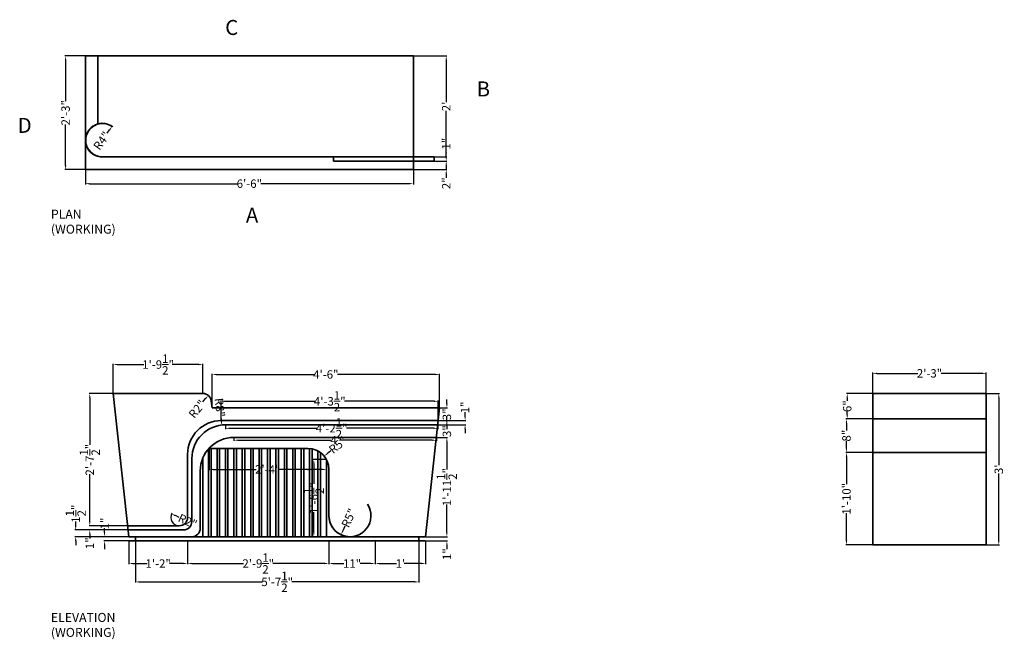
# Model space of a CAD drawing. Units: inches. Extents: x 461 to 695, y 519 to 666.
import ezdxf

# ---------------------------------------------------------------- set-up
doc = ezdxf.new("R2010")
doc.units = ezdxf.units.IN
doc.header["$MEASUREMENT"] = 0
for name, color, linetype, lineweight in [('A-ANNO-DIMS', 2, 'Continuous', 18), ('A-ANNO-TEXT', 3, 'Continuous', 25), ('A-FURN', 7, 'Continuous', 35)]:
    doc.layers.add(name, color=color, linetype=linetype, lineweight=lineweight)
doc.styles.get("Standard").update_dxf_attribs({"font": 'arial.ttf'})
doc.dimstyles.get("Standard").update_dxf_attribs({"dimtxt": 2, "dimasz": 1, "dimexe": 0.18, "dimexo": 0.0625, "dimgap": 0.09, "dimtad": 0, "dimdec": 1, "dimzin": 0, "dimdsep": 46, "dimlunit": 4, "dimtxsty": 'Standard', "dimcen": 0.09, "dimadec": 0, "dimazin": 0, "dimtfac": 1, "dimtdec": 1, "dimtofl": 0, "dimtmove": 0, "dimatfit": 3, "dimfxl": 1, "dimtolj": 1, "dimtzin": 0, "dimarcsym": 0})

# ---------------------------------------------------------------- blocks, each defined once
blk = doc.blocks.new('*D1')
at = {"layer": 'A-ANNO-DIMS', "color": 0, "lineweight": -2, "transparency": 16777216}
for p, q in [((562.35, 634.24), (562.35, 635.24)), ((559.57, 633.24), (562.53, 633.24)), ((559.57, 632.24), (562.53, 632.24)), ((562.35, 631.24), (562.35, 630.24))]:
    blk.add_line(p, q, dxfattribs=at)
at = {"layer": 'A-ANNO-DIMS', "color": 0, "transparency": 16777216}
for points in [[(562.18, 634.24), (562.51, 634.24), (562.35, 633.24)], [(562.18, 631.24), (562.51, 631.24), (562.35, 632.24)]]:
    blk.add_solid(points, dxfattribs=at)
at = {"layer": 'Defpoints', "color": 0, "transparency": 16777216}
for p in [(559.51, 633.24), (559.51, 632.24), (562.35, 633.24)]:
    blk.add_point(p, dxfattribs=at)
at = {"layer": 'A-ANNO-DIMS', "color": 0, "transparency": 16777216, "insert": (562.35, 636.39), "char_height": 2, "attachment_point": 5, "rotation": 90}
blk.add_mtext('\\A1;1"', dxfattribs=at)
blk = doc.blocks.new('*D2')
at = {"layer": 'A-ANNO-DIMS', "color": 0, "lineweight": -2, "transparency": 16777216}
for p, q in [((554.59, 632.24), (562.53, 632.24)), ((562.35, 633.24), (562.35, 634.24)), ((554.59, 630.24), (562.53, 630.24)), ((562.35, 629.24), (562.35, 628.24))]:
    blk.add_line(p, q, dxfattribs=at)
at = {"layer": 'A-ANNO-DIMS', "color": 0, "transparency": 16777216}
for points in [[(562.18, 633.24), (562.51, 633.24), (562.35, 632.24)], [(562.18, 629.24), (562.51, 629.24), (562.35, 630.24)]]:
    blk.add_solid(points, dxfattribs=at)
at = {"layer": 'Defpoints', "color": 0, "transparency": 16777216}
for p in [(554.53, 632.24), (554.53, 630.24), (562.35, 630.24)]:
    blk.add_point(p, dxfattribs=at)
at = {"layer": 'A-ANNO-DIMS', "color": 0, "transparency": 16777216, "insert": (562.35, 626.98), "char_height": 2, "attachment_point": 5, "rotation": 90}
blk.add_mtext('\\A1;2"', dxfattribs=at)
blk = doc.blocks.new('*D3')
at = {"layer": 'A-ANNO-DIMS', "color": 0, "lineweight": -2, "transparency": 16777216}
for p, q in [((554.59, 657.24), (562.53, 657.24)), ((562.35, 656.24), (562.35, 646.27)), ((562.35, 634.24), (562.35, 644.21)), ((554.59, 633.24), (562.53, 633.24))]:
    blk.add_line(p, q, dxfattribs=at)
at = {"layer": 'A-ANNO-DIMS', "color": 0, "transparency": 16777216}
for points in [[(562.18, 656.24), (562.51, 656.24), (562.35, 657.24)], [(562.18, 634.24), (562.51, 634.24), (562.35, 633.24)]]:
    blk.add_solid(points, dxfattribs=at)
at = {"layer": 'Defpoints', "color": 0, "transparency": 16777216}
for p in [(554.53, 657.24), (562.35, 657.24), (554.53, 633.24)]:
    blk.add_point(p, dxfattribs=at)
at = {"layer": 'A-ANNO-DIMS', "color": 0, "transparency": 16777216, "insert": (562.35, 645.24), "char_height": 2, "attachment_point": 5, "rotation": 90}
blk.add_mtext("\\A1;2'", dxfattribs=at)
blk = doc.blocks.new('*D4')
at = {"layer": 'A-ANNO-DIMS', "color": 0, "lineweight": -2, "transparency": 16777216}
for p, q in [((476.53, 630.18), (476.53, 626.7)), ((554.53, 630.18), (554.53, 626.7)), ((477.53, 626.88), (512.77, 626.88)), ((553.53, 626.88), (518.28, 626.88))]:
    blk.add_line(p, q, dxfattribs=at)
at = {"layer": 'A-ANNO-DIMS', "color": 0, "transparency": 16777216}
for points in [[(477.53, 627.04), (477.53, 626.71), (476.53, 626.88)], [(553.53, 627.04), (553.53, 626.71), (554.53, 626.88)]]:
    blk.add_solid(points, dxfattribs=at)
at = {"layer": 'Defpoints', "color": 0, "transparency": 16777216}
for p in [(476.53, 630.24), (554.53, 630.24), (476.53, 626.88)]:
    blk.add_point(p, dxfattribs=at)
at = {"layer": 'A-ANNO-DIMS', "color": 0, "transparency": 16777216, "insert": (515.53, 626.88), "char_height": 2, "attachment_point": 5}
blk.add_mtext('\\A1;6\'-6"', dxfattribs=at)
blk = doc.blocks.new('*D5')
at = {"layer": 'A-ANNO-DIMS', "color": 0, "lineweight": -2, "transparency": 16777216}
for p, q in [((476.46, 657.24), (471.65, 657.24)), ((471.83, 656.24), (471.83, 646.51)), ((471.83, 631.24), (471.83, 640.98)), ((476.46, 630.24), (471.65, 630.24))]:
    blk.add_line(p, q, dxfattribs=at)
at = {"layer": 'A-ANNO-DIMS', "color": 0, "transparency": 16777216}
for points in [[(471.66, 656.24), (472, 656.24), (471.83, 657.24)], [(471.66, 631.24), (472, 631.24), (471.83, 630.24)]]:
    blk.add_solid(points, dxfattribs=at)
at = {"layer": 'Defpoints', "color": 0, "transparency": 16777216}
for p in [(476.53, 657.24), (471.83, 630.24), (476.53, 630.24)]:
    blk.add_point(p, dxfattribs=at)
at = {"layer": 'A-ANNO-DIMS', "color": 0, "transparency": 16777216, "insert": (471.83, 643.74), "char_height": 2, "attachment_point": 5, "rotation": 90}
blk.add_mtext('\\A1;2\'-3"', dxfattribs=at)
blk = doc.blocks.new('*D6')
at = {"layer": 'A-ANNO-DIMS', "color": 0, "lineweight": -2, "transparency": 16777216}
blk.add_line((481.7, 638.86), (482.29, 639.67), dxfattribs=at)
blk.add_arc((480.53, 637.24), 4, 51.3987, 179.1048, dxfattribs=at)
at = {"layer": 'A-ANNO-DIMS', "color": 0, "transparency": 16777216}
blk.add_solid([(482.16, 639.76), (482.43, 639.57), (482.88, 640.48)], dxfattribs=at)
at = {"layer": 'Defpoints', "color": 0, "transparency": 16777216}
for p in [(482.88, 640.48), (480.53, 637.24)]:
    blk.add_point(p, dxfattribs=at)
at = {"layer": 'A-ANNO-DIMS', "color": 0, "transparency": 16777216, "insert": (480.41, 637.08), "char_height": 2, "attachment_point": 5, "rotation": 53.977}
blk.add_mtext('\\A1;R4"', dxfattribs=at)
blk = doc.blocks.new('*D7')
at = {"layer": 'A-ANNO-DIMS', "color": 0, "lineweight": -2, "transparency": 16777216}
for p, q in [((500.85, 541.88), (500.85, 536.4)), ((534.45, 541.88), (534.45, 536.4)), ((501.85, 536.58), (514.16, 536.58)), ((533.45, 536.58), (521.15, 536.58))]:
    blk.add_line(p, q, dxfattribs=at)
at = {"layer": 'A-ANNO-DIMS', "color": 0, "transparency": 16777216}
for points in [[(501.85, 536.74), (501.85, 536.41), (500.85, 536.58)], [(533.45, 536.74), (533.45, 536.41), (534.45, 536.58)]]:
    blk.add_solid(points, dxfattribs=at)
at = {"layer": 'Defpoints', "color": 0, "transparency": 16777216}
for p in [(500.85, 541.95), (534.45, 541.95), (534.45, 536.58)]:
    blk.add_point(p, dxfattribs=at)
at = {"layer": 'A-ANNO-DIMS', "color": 0, "transparency": 16777216, "insert": (517.65, 536.58), "char_height": 2, "attachment_point": 5}
blk.add_mtext('\\A1;2\'-9{\\H1x;\\S1/2;}"', dxfattribs=at)
blk = doc.blocks.new('*D8')
at = {"layer": 'A-ANNO-DIMS', "color": 0, "lineweight": -2, "transparency": 16777216}
for p, q in [((486.85, 541.88), (486.85, 536.4)), ((500.85, 541.88), (500.85, 536.4)), ((487.85, 536.58), (491.2, 536.58)), ((499.85, 536.58), (496.51, 536.58))]:
    blk.add_line(p, q, dxfattribs=at)
at = {"layer": 'A-ANNO-DIMS', "color": 0, "transparency": 16777216}
for points in [[(487.85, 536.74), (487.85, 536.41), (486.85, 536.58)], [(499.85, 536.74), (499.85, 536.41), (500.85, 536.58)]]:
    blk.add_solid(points, dxfattribs=at)
at = {"layer": 'Defpoints', "color": 0, "transparency": 16777216}
for p in [(486.85, 541.95), (500.85, 541.95), (500.85, 536.58)]:
    blk.add_point(p, dxfattribs=at)
at = {"layer": 'A-ANNO-DIMS', "color": 0, "transparency": 16777216, "insert": (493.85, 536.58), "char_height": 2, "attachment_point": 5}
blk.add_mtext('\\A1;1\'-2"', dxfattribs=at)
blk = doc.blocks.new('*D9')
at = {"layer": 'A-ANNO-DIMS', "color": 0, "lineweight": -2, "transparency": 16777216}
for p, q in [((534.45, 541.88), (534.45, 536.4)), ((545.45, 541.88), (545.45, 536.4)), ((535.45, 536.58), (538.03, 536.58)), ((544.45, 536.58), (541.87, 536.58))]:
    blk.add_line(p, q, dxfattribs=at)
at = {"layer": 'A-ANNO-DIMS', "color": 0, "transparency": 16777216}
for points in [[(535.45, 536.74), (535.45, 536.41), (534.45, 536.58)], [(544.45, 536.74), (544.45, 536.41), (545.45, 536.58)]]:
    blk.add_solid(points, dxfattribs=at)
at = {"layer": 'Defpoints', "color": 0, "transparency": 16777216}
for p in [(534.45, 541.95), (545.45, 541.95), (545.45, 536.58)]:
    blk.add_point(p, dxfattribs=at)
at = {"layer": 'A-ANNO-DIMS', "color": 0, "transparency": 16777216, "insert": (539.95, 536.58), "char_height": 2, "attachment_point": 5}
blk.add_mtext('\\A1;11"', dxfattribs=at)
blk = doc.blocks.new('*D10')
at = {"layer": 'A-ANNO-DIMS', "color": 0, "lineweight": -2, "transparency": 16777216}
for p, q in [((545.45, 541.88), (545.45, 536.4)), ((557.45, 541.88), (557.45, 536.4)), ((546.45, 536.58), (550.54, 536.58)), ((556.45, 536.58), (552.37, 536.58))]:
    blk.add_line(p, q, dxfattribs=at)
at = {"layer": 'A-ANNO-DIMS', "color": 0, "transparency": 16777216}
for points in [[(546.45, 536.74), (546.45, 536.41), (545.45, 536.58)], [(556.45, 536.74), (556.45, 536.41), (557.45, 536.58)]]:
    blk.add_solid(points, dxfattribs=at)
at = {"layer": 'Defpoints', "color": 0, "transparency": 16777216}
for p in [(545.45, 541.95), (557.45, 541.95), (557.45, 536.58)]:
    blk.add_point(p, dxfattribs=at)
at = {"layer": 'A-ANNO-DIMS', "color": 0, "transparency": 16777216, "insert": (551.45, 536.58), "char_height": 2, "attachment_point": 5}
blk.add_mtext("\\A1;1'", dxfattribs=at)
blk = doc.blocks.new('*D11')
at = {"layer": 'A-ANNO-DIMS', "color": 0, "lineweight": -2, "transparency": 16777216}
blk.add_line((498.85, 547.55), (497.94, 547.96), dxfattribs=at)
blk.add_arc((498.85, 547.55), 2, 150.5064, 268.2095, dxfattribs=at)
at = {"layer": 'A-ANNO-DIMS', "color": 0, "transparency": 16777216}
blk.add_solid([(498.01, 548.11), (497.87, 547.81), (497.03, 548.37)], dxfattribs=at)
at = {"layer": 'Defpoints', "color": 0, "transparency": 16777216}
for p in [(497.03, 548.37), (498.85, 547.55)]:
    blk.add_point(p, dxfattribs=at)
at = {"layer": 'A-ANNO-DIMS', "color": 0, "transparency": 16777216, "insert": (500.85, 546.64), "char_height": 2, "attachment_point": 5, "rotation": 335.663}
blk.add_mtext('\\A1;R2"', dxfattribs=at)
blk = doc.blocks.new('*D12')
at = {"layer": 'A-ANNO-DIMS', "color": 0, "lineweight": -2, "transparency": 16777216}
blk.add_line((538.27, 545.42), (537.76, 544.32), dxfattribs=at)
at = {"layer": 'A-ANNO-DIMS', "color": 0, "transparency": 16777216}
blk.add_solid([(537.61, 544.39), (537.91, 544.25), (537.34, 543.42)], dxfattribs=at)
at = {"layer": 'Defpoints', "color": 0, "transparency": 16777216}
for p in [(539.45, 547.95), (537.34, 543.42)]:
    blk.add_point(p, dxfattribs=at)
at = {"layer": 'A-ANNO-DIMS', "color": 0, "transparency": 16777216, "insert": (539.2, 547.41), "char_height": 2, "attachment_point": 5, "rotation": 65.0007}
blk.add_mtext('\\A1;R5"', dxfattribs=at)
blk = doc.blocks.new('*D13')
at = {"layer": 'A-ANNO-DIMS', "color": 0, "lineweight": -2, "transparency": 16777216}
for p, q in [((508.75, 571.49), (508.86, 570.49)), ((509.76, 561.55), (509.94, 561.55)), ((509.85, 561.46), (509.85, 561.64))]:
    blk.add_line(p, q, dxfattribs=at)
at = {"layer": 'A-ANNO-DIMS', "color": 0, "transparency": 16777216}
blk.add_solid([(509.02, 570.51), (508.69, 570.47), (508.97, 569.5)], dxfattribs=at)
at = {"layer": 'Defpoints', "color": 0, "transparency": 16777216}
for p in [(508.97, 569.5), (509.85, 561.55)]:
    blk.add_point(p, dxfattribs=at)
at = {"layer": 'A-ANNO-DIMS', "color": 0, "transparency": 16777216, "insert": (508.51, 573.67), "char_height": 2, "attachment_point": 5, "rotation": 276.3402}
blk.add_mtext('\\A1;R8"', dxfattribs=at)
blk = doc.blocks.new('*D14')
at = {"layer": 'A-ANNO-DIMS', "color": 0, "lineweight": -2, "transparency": 16777216}
blk.add_line((504.49, 575), (505.12, 575.78), dxfattribs=at)
at = {"layer": 'A-ANNO-DIMS', "color": 0, "transparency": 16777216}
blk.add_solid([(505, 575.88), (505.25, 575.67), (505.76, 576.55)], dxfattribs=at)
at = {"layer": 'Defpoints', "color": 0, "transparency": 16777216}
for p in [(505.76, 576.55), (504.49, 575)]:
    blk.add_point(p, dxfattribs=at)
at = {"layer": 'A-ANNO-DIMS', "color": 0, "transparency": 16777216, "insert": (503.11, 573.3), "char_height": 2, "attachment_point": 5, "rotation": 50.8113}
blk.add_mtext('\\A1;R2"', dxfattribs=at)
blk = doc.blocks.new('*D15')
at = {"layer": 'A-ANNO-DIMS', "color": 0, "lineweight": -2, "transparency": 16777216}
for p, q in [((534.89, 563.36), (534.11, 562.73)), ((529.36, 558.95), (529.54, 558.95)), ((529.45, 558.86), (529.45, 559.04))]:
    blk.add_line(p, q, dxfattribs=at)
at = {"layer": 'A-ANNO-DIMS', "color": 0, "transparency": 16777216}
blk.add_solid([(534, 562.86), (534.21, 562.6), (533.33, 562.1)], dxfattribs=at)
at = {"layer": 'Defpoints', "color": 0, "transparency": 16777216}
for p in [(533.33, 562.1), (529.45, 558.95)]:
    blk.add_point(p, dxfattribs=at)
at = {"layer": 'A-ANNO-DIMS', "color": 0, "transparency": 16777216, "insert": (536.59, 564.75), "char_height": 2, "attachment_point": 5, "rotation": 39.0868}
blk.add_mtext('\\A1;R5"', dxfattribs=at)
blk = doc.blocks.new('*D16')
at = {"layer": 'A-ANNO-DIMS', "color": 0, "lineweight": -2, "transparency": 16777216}
for p, q in [((506.66, 573.61), (506.66, 581.7)), ((507.66, 581.52), (530.93, 581.52)), ((559.78, 581.52), (536.51, 581.52)), ((560.78, 573.61), (560.78, 581.7))]:
    blk.add_line(p, q, dxfattribs=at)
at = {"layer": 'A-ANNO-DIMS', "color": 0, "transparency": 16777216}
for points in [[(507.66, 581.68), (507.66, 581.35), (506.66, 581.52)], [(559.78, 581.68), (559.78, 581.35), (560.78, 581.52)]]:
    blk.add_solid(points, dxfattribs=at)
at = {"layer": 'Defpoints', "color": 0, "transparency": 16777216}
for p in [(506.66, 581.52), (506.66, 573.55), (560.78, 573.55)]:
    blk.add_point(p, dxfattribs=at)
at = {"layer": 'A-ANNO-DIMS', "color": 0, "transparency": 16777216, "insert": (533.72, 581.52), "char_height": 2, "attachment_point": 5}
blk.add_mtext('\\A1;4\'-6"', dxfattribs=at)
blk = doc.blocks.new('*D17')
at = {"layer": 'A-ANNO-DIMS', "color": 0, "lineweight": -2, "transparency": 16777216}
for p, q in [((483.15, 577.06), (483.15, 584.06)), ((484.15, 583.88), (490.44, 583.88)), ((503.49, 583.88), (497.21, 583.88)), ((504.49, 577.06), (504.49, 584.06))]:
    blk.add_line(p, q, dxfattribs=at)
at = {"layer": 'A-ANNO-DIMS', "color": 0, "transparency": 16777216}
for points in [[(484.15, 584.05), (484.15, 583.72), (483.15, 583.88)], [(503.49, 584.05), (503.49, 583.72), (504.49, 583.88)]]:
    blk.add_solid(points, dxfattribs=at)
at = {"layer": 'Defpoints', "color": 0, "transparency": 16777216}
for p in [(504.49, 583.88), (483.15, 577), (504.49, 577)]:
    blk.add_point(p, dxfattribs=at)
at = {"layer": 'A-ANNO-DIMS', "color": 0, "transparency": 16777216, "insert": (493.82, 583.88), "char_height": 2, "attachment_point": 5}
blk.add_mtext('\\A1;1\'-9{\\H1x;\\S1/2;}"', dxfattribs=at)
blk = doc.blocks.new('*D18')
at = {"layer": 'A-ANNO-DIMS', "color": 0, "lineweight": -2, "transparency": 16777216}
for p, q in [((562.5, 543.95), (562.5, 544.95)), ((557.41, 541.95), (562.68, 541.95)), ((557.51, 542.95), (562.68, 542.95)), ((562.5, 540.95), (562.5, 539.95))]:
    blk.add_line(p, q, dxfattribs=at)
at = {"layer": 'A-ANNO-DIMS', "color": 0, "transparency": 16777216}
for points in [[(562.34, 543.95), (562.67, 543.95), (562.5, 542.95)], [(562.34, 540.95), (562.67, 540.95), (562.5, 541.95)]]:
    blk.add_solid(points, dxfattribs=at)
at = {"layer": 'Defpoints', "color": 0, "transparency": 16777216}
for p in [(557.34, 541.95), (557.45, 542.95), (562.5, 541.95)]:
    blk.add_point(p, dxfattribs=at)
at = {"layer": 'A-ANNO-DIMS', "color": 0, "transparency": 16777216, "insert": (562.5, 538.8), "char_height": 2, "attachment_point": 5, "rotation": 90}
blk.add_mtext('\\A1;1"', dxfattribs=at)
blk = doc.blocks.new('*D19')
at = {"layer": 'A-ANNO-DIMS', "color": 0, "lineweight": -2, "transparency": 16777216}
for p, q in [((560.08, 566.55), (562.68, 566.55)), ((562.5, 565.55), (562.5, 558.91)), ((562.5, 543.95), (562.5, 550.59)), ((557.51, 542.95), (562.68, 542.95))]:
    blk.add_line(p, q, dxfattribs=at)
at = {"layer": 'A-ANNO-DIMS', "color": 0, "transparency": 16777216}
for points in [[(562.34, 565.55), (562.67, 565.55), (562.5, 566.55)], [(562.34, 543.95), (562.67, 543.95), (562.5, 542.95)]]:
    blk.add_solid(points, dxfattribs=at)
at = {"layer": 'Defpoints', "color": 0, "transparency": 16777216}
for p in [(560.02, 566.55), (562.5, 566.55), (557.45, 542.95)]:
    blk.add_point(p, dxfattribs=at)
at = {"layer": 'A-ANNO-DIMS', "color": 0, "transparency": 16777216, "insert": (562.5, 554.75), "char_height": 2, "attachment_point": 5, "rotation": 90}
blk.add_mtext('\\A1;1\'-11{\\H1x;\\S1/2;}"', dxfattribs=at)
blk = doc.blocks.new('*D20')
at = {"layer": 'A-ANNO-DIMS', "color": 0, "lineweight": -2, "transparency": 16777216}
for p, q in [((562.5, 570.55), (562.5, 571.55)), ((560.4, 569.55), (562.68, 569.55)), ((560.08, 566.55), (562.68, 566.55)), ((562.5, 565.55), (562.5, 564.55))]:
    blk.add_line(p, q, dxfattribs=at)
at = {"layer": 'A-ANNO-DIMS', "color": 0, "transparency": 16777216}
for points in [[(562.34, 570.55), (562.67, 570.55), (562.5, 569.55)], [(562.34, 565.55), (562.67, 565.55), (562.5, 566.55)]]:
    blk.add_solid(points, dxfattribs=at)
at = {"layer": 'Defpoints', "color": 0, "transparency": 16777216}
for p in [(560.34, 569.55), (560.02, 566.55), (562.5, 566.55)]:
    blk.add_point(p, dxfattribs=at)
at = {"layer": 'A-ANNO-DIMS', "color": 0, "transparency": 16777216, "insert": (562.5, 568.05), "char_height": 2, "attachment_point": 5, "rotation": 90}
blk.add_mtext('\\A1;3"', dxfattribs=at)
blk = doc.blocks.new('*D21')
at = {"layer": 'A-ANNO-DIMS', "color": 0, "lineweight": -2, "transparency": 16777216}
for p, q in [((566.83, 571.55), (566.83, 572.55)), ((560.4, 569.55), (567.01, 569.55)), ((560.51, 570.55), (567.01, 570.55)), ((566.83, 568.55), (566.83, 567.55))]:
    blk.add_line(p, q, dxfattribs=at)
at = {"layer": 'A-ANNO-DIMS', "color": 0, "transparency": 16777216}
for points in [[(566.67, 571.55), (567, 571.55), (566.83, 570.55)], [(566.67, 568.55), (567, 568.55), (566.83, 569.55)]]:
    blk.add_solid(points, dxfattribs=at)
at = {"layer": 'Defpoints', "color": 0, "transparency": 16777216}
for p in [(560.34, 569.55), (560.45, 570.55), (566.83, 570.55)]:
    blk.add_point(p, dxfattribs=at)
at = {"layer": 'A-ANNO-DIMS', "color": 0, "transparency": 16777216, "insert": (566.83, 573.69), "char_height": 2, "attachment_point": 5, "rotation": 90}
blk.add_mtext('\\A1;1"', dxfattribs=at)
blk = doc.blocks.new('*D22')
at = {"layer": 'A-ANNO-DIMS', "color": 0, "lineweight": -2, "transparency": 16777216}
for p, q in [((562.5, 574.55), (562.5, 575.55)), ((560.84, 573.55), (562.68, 573.55)), ((560.51, 570.55), (562.68, 570.55)), ((562.5, 569.55), (562.5, 568.55))]:
    blk.add_line(p, q, dxfattribs=at)
at = {"layer": 'A-ANNO-DIMS', "color": 0, "transparency": 16777216}
for points in [[(562.34, 574.55), (562.67, 574.55), (562.5, 573.55)], [(562.34, 569.55), (562.67, 569.55), (562.5, 570.55)]]:
    blk.add_solid(points, dxfattribs=at)
at = {"layer": 'Defpoints', "color": 0, "transparency": 16777216}
for p in [(560.78, 573.55), (560.45, 570.55), (562.5, 570.55)]:
    blk.add_point(p, dxfattribs=at)
at = {"layer": 'A-ANNO-DIMS', "color": 0, "transparency": 16777216, "insert": (562.5, 572.05), "char_height": 2, "attachment_point": 5, "rotation": 90}
blk.add_mtext('\\A1;3"', dxfattribs=at)
blk = doc.blocks.new('*D23')
at = {"layer": 'A-ANNO-DIMS', "color": 0, "lineweight": -2, "transparency": 16777216}
for p, q in [((481.09, 543.95), (481.09, 544.95)), ((486.79, 542.95), (480.91, 542.95)), ((486.9, 541.95), (480.91, 541.95)), ((481.09, 540.95), (481.09, 539.95))]:
    blk.add_line(p, q, dxfattribs=at)
at = {"layer": 'A-ANNO-DIMS', "color": 0, "transparency": 16777216}
for points in [[(480.93, 543.95), (481.26, 543.95), (481.09, 542.95)], [(480.93, 540.95), (481.26, 540.95), (481.09, 541.95)]]:
    blk.add_solid(points, dxfattribs=at)
at = {"layer": 'Defpoints', "color": 0, "transparency": 16777216}
for p in [(481.09, 542.95), (486.85, 542.95), (486.96, 541.95)]:
    blk.add_point(p, dxfattribs=at)
at = {"layer": 'A-ANNO-DIMS', "color": 0, "transparency": 16777216, "insert": (481.09, 546.09), "char_height": 2, "attachment_point": 5, "rotation": 90}
blk.add_mtext('\\A1;1"', dxfattribs=at)
blk = doc.blocks.new('*D24')
at = {"layer": 'A-ANNO-DIMS', "color": 0, "lineweight": -2, "transparency": 16777216}
for p, q in [((474.23, 545.55), (474.23, 546.55)), ((486.62, 544.55), (474.05, 544.55)), ((486.79, 542.95), (474.05, 542.95)), ((474.23, 541.95), (474.23, 540.95))]:
    blk.add_line(p, q, dxfattribs=at)
at = {"layer": 'A-ANNO-DIMS', "color": 0, "transparency": 16777216}
for points in [[(474.06, 545.55), (474.4, 545.55), (474.23, 544.55)], [(474.06, 541.95), (474.4, 541.95), (474.23, 542.95)]]:
    blk.add_solid(points, dxfattribs=at)
at = {"layer": 'Defpoints', "color": 0, "transparency": 16777216}
for p in [(474.23, 544.55), (486.68, 544.55), (486.85, 542.95)]:
    blk.add_point(p, dxfattribs=at)
at = {"layer": 'A-ANNO-DIMS', "color": 0, "transparency": 16777216, "insert": (474.23, 548.42), "char_height": 2, "attachment_point": 5, "rotation": 90}
blk.add_mtext('\\A1;1{\\H1x;\\S1/2;}"', dxfattribs=at)
blk = doc.blocks.new('*D25')
at = {"layer": 'A-ANNO-DIMS', "color": 0, "lineweight": -2, "transparency": 16777216}
for p, q in [((477.58, 546.55), (477.58, 547.55)), ((486.51, 545.55), (477.4, 545.55)), ((486.62, 544.55), (477.4, 544.55)), ((477.58, 543.55), (477.58, 542.55))]:
    blk.add_line(p, q, dxfattribs=at)
at = {"layer": 'A-ANNO-DIMS', "color": 0, "transparency": 16777216}
for points in [[(477.41, 546.55), (477.74, 546.55), (477.58, 545.55)], [(477.41, 543.55), (477.74, 543.55), (477.58, 544.55)]]:
    blk.add_solid(points, dxfattribs=at)
at = {"layer": 'Defpoints', "color": 0, "transparency": 16777216}
for p in [(477.58, 544.55), (486.57, 545.55), (486.68, 544.55)]:
    blk.add_point(p, dxfattribs=at)
at = {"layer": 'A-ANNO-DIMS', "color": 0, "transparency": 16777216, "insert": (477.58, 541.4), "char_height": 2, "attachment_point": 5, "rotation": 90}
blk.add_mtext('\\A1;1"', dxfattribs=at)
blk = doc.blocks.new('*D26')
at = {"layer": 'A-ANNO-DIMS', "color": 0, "lineweight": -2, "transparency": 16777216}
for p, q in [((483.09, 577), (477.4, 577)), ((477.58, 576), (477.58, 564.77)), ((477.58, 546.55), (477.58, 557.78)), ((486.51, 545.55), (477.4, 545.55))]:
    blk.add_line(p, q, dxfattribs=at)
at = {"layer": 'A-ANNO-DIMS', "color": 0, "transparency": 16777216}
for points in [[(477.41, 576), (477.74, 576), (477.58, 577)], [(477.41, 546.55), (477.74, 546.55), (477.58, 545.55)]]:
    blk.add_solid(points, dxfattribs=at)
at = {"layer": 'Defpoints', "color": 0, "transparency": 16777216}
for p in [(477.58, 577), (483.15, 577), (486.57, 545.55)]:
    blk.add_point(p, dxfattribs=at)
at = {"layer": 'A-ANNO-DIMS', "color": 0, "transparency": 16777216, "insert": (477.58, 561.27), "char_height": 2, "attachment_point": 5, "rotation": 90}
blk.add_mtext('\\A1;2\'-7{\\H1x;\\S1/2;}"', dxfattribs=at)
blk = doc.blocks.new('*D27')
at = {"layer": 'A-ANNO-DIMS', "color": 0, "lineweight": -2, "transparency": 16777216}
for p, q in [((663.72, 576.98), (657.53, 576.98)), ((657.71, 575.98), (657.71, 575.23)), ((657.71, 571.98), (657.71, 572.74)), ((663.72, 570.98), (657.53, 570.98))]:
    blk.add_line(p, q, dxfattribs=at)
at = {"layer": 'A-ANNO-DIMS', "color": 0, "transparency": 16777216}
for points in [[(657.54, 575.98), (657.88, 575.98), (657.71, 576.98)], [(657.54, 571.98), (657.88, 571.98), (657.71, 570.98)]]:
    blk.add_solid(points, dxfattribs=at)
at = {"layer": 'Defpoints', "color": 0, "transparency": 16777216}
for p in [(663.78, 576.98), (657.71, 570.98), (663.78, 570.98)]:
    blk.add_point(p, dxfattribs=at)
at = {"layer": 'A-ANNO-DIMS', "color": 0, "transparency": 16777216, "insert": (657.71, 573.98), "char_height": 2, "attachment_point": 5, "rotation": 90}
blk.add_mtext('\\A1;6"', dxfattribs=at)
blk = doc.blocks.new('*D28')
at = {"layer": 'A-ANNO-DIMS', "color": 0, "lineweight": -2, "transparency": 16777216}
for p, q in [((663.72, 570.98), (657.35, 570.98)), ((657.53, 569.98), (657.53, 568.22)), ((657.53, 563.98), (657.53, 565.74)), ((663.72, 562.98), (657.35, 562.98))]:
    blk.add_line(p, q, dxfattribs=at)
at = {"layer": 'A-ANNO-DIMS', "color": 0, "transparency": 16777216}
for points in [[(657.36, 569.98), (657.7, 569.98), (657.53, 570.98)], [(657.36, 563.98), (657.7, 563.98), (657.53, 562.98)]]:
    blk.add_solid(points, dxfattribs=at)
at = {"layer": 'Defpoints', "color": 0, "transparency": 16777216}
for p in [(663.78, 570.98), (657.53, 562.98), (663.78, 562.98)]:
    blk.add_point(p, dxfattribs=at)
at = {"layer": 'A-ANNO-DIMS', "color": 0, "transparency": 16777216, "insert": (657.53, 566.98), "char_height": 2, "attachment_point": 5, "rotation": 90}
blk.add_mtext('\\A1;8"', dxfattribs=at)
blk = doc.blocks.new('*D29')
at = {"layer": 'A-ANNO-DIMS', "color": 0, "lineweight": -2, "transparency": 16777216}
for p, q in [((663.72, 562.98), (657.35, 562.98)), ((657.53, 561.98), (657.53, 555.41)), ((657.53, 541.98), (657.53, 548.55)), ((663.72, 540.98), (657.35, 540.98))]:
    blk.add_line(p, q, dxfattribs=at)
at = {"layer": 'A-ANNO-DIMS', "color": 0, "transparency": 16777216}
for points in [[(657.36, 561.98), (657.7, 561.98), (657.53, 562.98)], [(657.36, 541.98), (657.7, 541.98), (657.53, 540.98)]]:
    blk.add_solid(points, dxfattribs=at)
at = {"layer": 'Defpoints', "color": 0, "transparency": 16777216}
for p in [(663.78, 562.98), (657.53, 540.98), (663.78, 540.98)]:
    blk.add_point(p, dxfattribs=at)
at = {"layer": 'A-ANNO-DIMS', "color": 0, "transparency": 16777216, "insert": (657.53, 551.98), "char_height": 2, "attachment_point": 5, "rotation": 90}
blk.add_mtext('\\A1;1\'-10"', dxfattribs=at)
blk = doc.blocks.new('*D30')
at = {"layer": 'A-ANNO-DIMS', "color": 0, "lineweight": -2, "transparency": 16777216}
for p, q in [((663.78, 577.05), (663.78, 581.97)), ((664.78, 581.79), (674.52, 581.79)), ((689.78, 581.79), (680.05, 581.79)), ((690.78, 577.05), (690.78, 581.97))]:
    blk.add_line(p, q, dxfattribs=at)
at = {"layer": 'A-ANNO-DIMS', "color": 0, "transparency": 16777216}
for points in [[(664.78, 581.95), (664.78, 581.62), (663.78, 581.79)], [(689.78, 581.95), (689.78, 581.62), (690.78, 581.79)]]:
    blk.add_solid(points, dxfattribs=at)
at = {"layer": 'Defpoints', "color": 0, "transparency": 16777216}
for p in [(663.78, 581.79), (663.78, 576.98), (690.78, 576.98)]:
    blk.add_point(p, dxfattribs=at)
at = {"layer": 'A-ANNO-DIMS', "color": 0, "transparency": 16777216, "insert": (677.28, 581.79), "char_height": 2, "attachment_point": 5}
blk.add_mtext('\\A1;2\'-3"', dxfattribs=at)
blk = doc.blocks.new('*D31')
at = {"layer": 'A-ANNO-DIMS', "color": 0, "lineweight": -2, "transparency": 16777216}
for p, q in [((690.85, 576.98), (693.94, 576.98)), ((693.76, 575.98), (693.76, 559.99)), ((693.76, 541.98), (693.76, 557.97)), ((690.85, 540.98), (693.94, 540.98))]:
    blk.add_line(p, q, dxfattribs=at)
at = {"layer": 'A-ANNO-DIMS', "color": 0, "transparency": 16777216}
for points in [[(693.59, 575.98), (693.92, 575.98), (693.76, 576.98)], [(693.59, 541.98), (693.92, 541.98), (693.76, 540.98)]]:
    blk.add_solid(points, dxfattribs=at)
at = {"layer": 'Defpoints', "color": 0, "transparency": 16777216}
for p in [(690.78, 576.98), (693.76, 576.98), (690.78, 540.98)]:
    blk.add_point(p, dxfattribs=at)
at = {"layer": 'A-ANNO-DIMS', "color": 0, "transparency": 16777216, "insert": (693.76, 558.98), "char_height": 2, "attachment_point": 5, "rotation": 90}
blk.add_mtext("\\A1;3'", dxfattribs=at)
blk = doc.blocks.new('*D32')
at = {"layer": 'A-ANNO-DIMS', "color": 0, "lineweight": -2, "transparency": 16777216}
for p, q in [((488.45, 541.88), (488.45, 532.03)), ((555.85, 541.88), (555.85, 532.03)), ((489.45, 532.21), (518.67, 532.21)), ((554.85, 532.21), (525.63, 532.21))]:
    blk.add_line(p, q, dxfattribs=at)
at = {"layer": 'A-ANNO-DIMS', "color": 0, "transparency": 16777216}
for points in [[(489.45, 532.37), (489.45, 532.04), (488.45, 532.21)], [(554.85, 532.37), (554.85, 532.04), (555.85, 532.21)]]:
    blk.add_solid(points, dxfattribs=at)
at = {"layer": 'Defpoints', "color": 0, "transparency": 16777216}
for p in [(488.45, 541.95), (555.85, 541.95), (555.85, 532.21)]:
    blk.add_point(p, dxfattribs=at)
at = {"layer": 'A-ANNO-DIMS', "color": 0, "transparency": 16777216, "insert": (522.15, 532.21), "char_height": 2, "attachment_point": 5}
blk.add_mtext('\\A1;5\'-7{\\H1x;\\S1/2;}"', dxfattribs=at)
blk = doc.blocks.new('*D33')
at = {"layer": 'A-ANNO-DIMS', "color": 0, "lineweight": -2, "transparency": 16777216}
for p, q in [((505.95, 563.88), (505.95, 558.77)), ((533.85, 561.26), (533.85, 558.77)), ((506.95, 558.95), (517.14, 558.95)), ((532.85, 558.95), (522.67, 558.95))]:
    blk.add_line(p, q, dxfattribs=at)
at = {"layer": 'A-ANNO-DIMS', "color": 0, "transparency": 16777216}
for points in [[(506.95, 559.11), (506.95, 558.78), (505.95, 558.95)], [(532.85, 559.11), (532.85, 558.78), (533.85, 558.95)]]:
    blk.add_solid(points, dxfattribs=at)
at = {"layer": 'Defpoints', "color": 0, "transparency": 16777216}
for p in [(505.95, 563.95), (533.85, 561.32), (533.85, 558.95)]:
    blk.add_point(p, dxfattribs=at)
at = {"layer": 'A-ANNO-DIMS', "color": 0, "transparency": 16777216, "insert": (519.9, 558.95), "char_height": 2, "attachment_point": 5}
blk.add_mtext('\\A1;2\'-4"', dxfattribs=at)
blk = doc.blocks.new('*D34')
at = {"layer": 'A-ANNO-DIMS', "color": 0, "lineweight": -2, "transparency": 16777216}
for p, q in [((533.79, 561.32), (530.68, 561.32)), ((530.86, 560.32), (530.86, 555.52)), ((530.86, 543.95), (530.86, 548.75)), ((533.79, 542.95), (530.68, 542.95))]:
    blk.add_line(p, q, dxfattribs=at)
at = {"layer": 'A-ANNO-DIMS', "color": 0, "transparency": 16777216}
for points in [[(530.7, 560.32), (531.03, 560.32), (530.86, 561.32)], [(530.7, 543.95), (531.03, 543.95), (530.86, 542.95)]]:
    blk.add_solid(points, dxfattribs=at)
at = {"layer": 'Defpoints', "color": 0, "transparency": 16777216}
for p in [(533.85, 561.32), (530.86, 542.95), (533.85, 542.95)]:
    blk.add_point(p, dxfattribs=at)
at = {"layer": 'A-ANNO-DIMS', "color": 0, "transparency": 16777216, "insert": (530.86, 552.13), "char_height": 2, "attachment_point": 5, "rotation": 90}
blk.add_mtext('\\A1;1\'-6{\\H1x;\\S1/2;}"', dxfattribs=at)
blk = doc.blocks.new('*D35')
at = {"layer": 'A-ANNO-DIMS', "color": 0, "lineweight": -2, "transparency": 16777216}
for p, q in [((509.85, 569.48), (509.85, 568.55)), ((560.34, 569.48), (560.34, 568.55)), ((510.85, 568.73), (531.58, 568.73)), ((559.34, 568.73), (538.61, 568.73))]:
    blk.add_line(p, q, dxfattribs=at)
at = {"layer": 'A-ANNO-DIMS', "color": 0, "transparency": 16777216}
for points in [[(510.85, 568.89), (510.85, 568.56), (509.85, 568.73)], [(559.34, 568.89), (559.34, 568.56), (560.34, 568.73)]]:
    blk.add_solid(points, dxfattribs=at)
at = {"layer": 'Defpoints', "color": 0, "transparency": 16777216}
for p in [(509.85, 569.55), (560.34, 569.55), (509.85, 568.73)]:
    blk.add_point(p, dxfattribs=at)
at = {"layer": 'A-ANNO-DIMS', "color": 0, "transparency": 16777216, "insert": (535.1, 568.73), "char_height": 2, "attachment_point": 5}
blk.add_mtext('\\A1;4\'-2{\\H1x;\\S1/2;}"', dxfattribs=at)
blk = doc.blocks.new('*D36')
at = {"layer": 'A-ANNO-DIMS', "color": 0, "lineweight": -2, "transparency": 16777216}
for p, q in [((511.85, 566.48), (511.85, 565.71)), ((512.85, 565.89), (534.88, 565.89)), ((559.02, 565.89), (536.98, 565.89)), ((560.02, 566.48), (560.02, 565.71))]:
    blk.add_line(p, q, dxfattribs=at)
at = {"layer": 'A-ANNO-DIMS', "color": 0, "transparency": 16777216}
for points in [[(512.85, 566.05), (512.85, 565.72), (511.85, 565.89)], [(559.02, 566.05), (559.02, 565.72), (560.02, 565.89)]]:
    blk.add_solid(points, dxfattribs=at)
at = {"layer": 'Defpoints', "color": 0, "transparency": 16777216}
for p in [(511.85, 566.55), (511.85, 565.89), (560.02, 566.55)]:
    blk.add_point(p, dxfattribs=at)
at = {"layer": 'A-ANNO-DIMS', "color": 0, "transparency": 16777216, "insert": (535.93, 565.89), "char_height": 2, "attachment_point": 5}
blk.add_mtext("\\A1;4'", dxfattribs=at)
blk = doc.blocks.new('*D37')
at = {"layer": 'A-ANNO-DIMS', "color": 0, "lineweight": -2, "transparency": 16777216}
for p, q in [((508.85, 570.61), (508.85, 575.32)), ((509.85, 575.14), (531.13, 575.14)), ((559.45, 575.14), (538.17, 575.14)), ((560.45, 570.61), (560.45, 575.32))]:
    blk.add_line(p, q, dxfattribs=at)
at = {"layer": 'A-ANNO-DIMS', "color": 0, "transparency": 16777216}
for points in [[(509.85, 575.31), (509.85, 574.97), (508.85, 575.14)], [(559.45, 575.31), (559.45, 574.97), (560.45, 575.14)]]:
    blk.add_solid(points, dxfattribs=at)
at = {"layer": 'Defpoints', "color": 0, "transparency": 16777216}
for p in [(508.85, 575.14), (508.85, 570.55), (560.45, 570.55)]:
    blk.add_point(p, dxfattribs=at)
at = {"layer": 'A-ANNO-DIMS', "color": 0, "transparency": 16777216, "insert": (534.65, 575.14), "char_height": 2, "attachment_point": 5}
blk.add_mtext('\\A1;4\'-3{\\H1x;\\S1/2;}"', dxfattribs=at)

msp = doc.modelspace()

# ---------------------------------------------------------------- linework, layer by layer
at = {"layer": 'A-FURN'}
for p, q in [((476.53, 657.24), (554.53, 657.24)), ((476.53, 637.24), (476.53, 657.24)), ((479.53, 641.06), (479.53, 657.24)), ((554.53, 657.24), (554.53, 633.24)), ((476.53, 630.24), (476.53, 637.24)), ((554.53, 633.24), (480.53, 633.24)), ((554.53, 633.24), (554.53, 630.24)), ((554.53, 630.24), (476.53, 630.24)), ((483.15, 577), (504.49, 577)), ((486.85, 542.95), (483.15, 577)), ((690.78, 576.98), (663.78, 576.98)), ((663.78, 576.98), (663.78, 570.98)), ((690.78, 540.98), (690.78, 576.98)), ((506.66, 573.55), (506.48, 575.22)), ((560.78, 573.55), (506.66, 573.55)), ((557.45, 542.95), (560.78, 573.55)), ((560.45, 570.55), (508.85, 570.55)), ((560.34, 569.55), (509.85, 569.55)), ((663.78, 570.98), (663.78, 562.98)), ((663.78, 570.98), (690.78, 570.98)), ((560.02, 566.55), (511.85, 566.55)), ((500.85, 547.55), (500.85, 562.55)), ((505.85, 563.84), (505.85, 542.95)), ((505.95, 563.95), (529.45, 563.95)), ((506.45, 563.95), (506.45, 542.95)), ((507.85, 563.95), (507.85, 542.95)), ((508.45, 563.95), (508.45, 542.95)), ((509.85, 563.95), (509.85, 542.95)), ((510.45, 563.95), (510.45, 542.95)), ((511.85, 563.95), (511.85, 542.95)), ((512.45, 563.95), (512.45, 542.95)), ((513.85, 563.95), (513.85, 542.95)), ((514.45, 563.95), (514.45, 542.95)), ((515.85, 563.95), (515.85, 542.95)), ((516.45, 563.95), (516.45, 542.95)), ((517.85, 563.95), (517.85, 542.95)), ((518.45, 563.95), (518.45, 542.95)), ((519.85, 563.95), (519.85, 542.95)), ((520.45, 563.95), (520.45, 542.95)), ((521.85, 563.95), (521.85, 542.95)), ((522.45, 563.95), (522.45, 542.95)), ((523.85, 563.95), (523.85, 542.95)), ((524.45, 563.95), (524.45, 542.95)), ((525.85, 563.95), (525.85, 542.95)), ((526.45, 563.95), (526.45, 542.95)), ((527.85, 563.95), (527.85, 542.95)), ((528.45, 563.95), (528.45, 542.95)), ((529.85, 563.93), (529.85, 542.95)), ((530.45, 563.85), (530.45, 542.95)), ((531.85, 563.33), (531.85, 542.95)), ((532.45, 562.95), (532.45, 542.95)), ((663.78, 562.98), (663.78, 540.98)), ((663.78, 562.98), (690.78, 562.98)), ((501.85, 546.55), (501.85, 561.55)), ((504.45, 561.59), (504.45, 542.95)), ((533.85, 561.32), (533.85, 542.95)), ((503.85, 544.95), (503.85, 558.55)), ((534.45, 547.95), (534.45, 558.95)), ((486.57, 545.55), (498.85, 545.55)), ((486.68, 544.55), (499.85, 544.55)), ((486.85, 542.95), (501.85, 542.95)), ((486.85, 541.95), (500.85, 541.95)), ((488.45, 542.95), (488.45, 541.95)), ((500.85, 541.95), (534.45, 541.95)), ((501.85, 542.95), (539.45, 542.95)), ((534.45, 541.95), (545.45, 541.95)), ((539.45, 542.95), (557.45, 542.95)), ((545.45, 541.95), (557.34, 541.95)), ((555.85, 542.95), (555.85, 541.95)), ((663.78, 540.98), (690.78, 540.98))]:
    msp.add_line(p, q, dxfattribs=at)
msp.add_lwpolyline([(535.51, 632.24), (559.51, 632.24), (559.51, 633.24), (535.51, 633.24)], close=True, dxfattribs=at)
for centre, radius, start, end in [((480.59, 637.22), 3.98, 54.8081, 270.8311), ((480.53, 637.24), 4, 180, 270), ((504.49, 575), 2, 6.201, 90), ((508.85, 562.55), 8, 90, 180), ((509.85, 561.55), 8, 90, 180), ((511.85, 558.55), 8, 90, 180), ((529.45, 558.95), 5, 0, 90), ((539.45, 547.95), 5, 180, 33.3084), ((539.45, 547.95), 5, 180, 270), ((498.85, 547.55), 2, 270, 0), ((499.85, 546.55), 2, 270, 0), ((501.85, 544.95), 2, 270, 0)]:
    msp.add_arc(centre, radius, start, end, dxfattribs=at)

# ---------------------------------------------------------------- texts
at = {"layer": 'A-ANNO-TEXT', "attachment_point": 1}
for s, width, gutter_width, insert, char_height in [('C', 131.4437, 17.85, (509.78, 665.8), 3.57), ('B', 131.4437, 17.85, (569.57, 651.19), 3.57), ('D', 131.4437, 17.85, (460.42, 642.53), 3.57), ('PLAN\\P(WORKING)', 1266.6755, 10.68, (468.34, 620.69), 2.137), ('A', 131.4437, 17.85, (514.7, 621.17), 3.57), ('ELEVATION\\P(WORKING)', 1266.6755, 10.68, (468.34, 524.83), 2.137)]:
    msp.add_mtext_dynamic_manual_height_columns(s, width=width, gutter_width=gutter_width, heights=[0], dxfattribs=dict(at, insert=insert, char_height=char_height))

# ---------------------------------------------------------------- dimensions: what is measured, and where the dimension line sits
at = {"layer": 'A-ANNO-DIMS'}
for base, p1, p2, picture, middle in [((471.83, 630.24), (476.53, 657.24), (476.53, 630.24), '*D5', (471.83, 643.74)), ((562.35, 657.24), (554.53, 633.24), (554.53, 657.24), '*D3', (562.35, 645.24)), ((562.35, 633.24), (559.51, 632.24), (559.51, 633.24), '*D1', (562.35, 636.39)), ((562.35, 630.24), (554.53, 632.24), (554.53, 630.24), '*D2', (562.35, 626.98)), ((477.5763, 577.0005), (486.5696, 545.5471), (483.1521, 577.0005), '*D26', (477.5763, 561.2738)), ((657.71, 570.98), (663.78, 576.98), (663.78, 570.98), '*D27', (657.71, 573.98)), ((693.76, 576.98), (690.78, 540.98), (690.78, 576.98), '*D31', (693.76, 558.98)), ((566.83, 570.55), (560.34, 569.55), (560.45, 570.55), '*D21', (566.83, 573.69)), ((562.5, 570.55), (560.78, 573.55), (560.45, 570.55), '*D22', (562.5, 572.05)), ((562.5, 566.55), (560.34, 569.55), (560.02, 566.55), '*D20', (562.5, 568.05)), ((657.53, 562.98), (663.78, 570.98), (663.78, 562.98), '*D28', (657.53, 566.98)), ((562.5, 566.55), (557.45, 542.95), (560.02, 566.55), '*D19', (562.5, 554.75)), ((657.53, 540.98), (663.78, 562.98), (663.78, 540.98), '*D29', (657.53, 551.98)), ((530.86, 542.95), (533.85, 561.32), (533.85, 542.95), '*D34', (530.86, 552.13)), ((474.23, 544.55), (486.85, 542.95), (486.68, 544.55), '*D24', (474.23, 548.42)), ((477.58, 544.55), (486.57, 545.55), (486.68, 544.55), '*D25', (477.58, 541.4)), ((481.09, 542.95), (486.96, 541.95), (486.85, 542.95), '*D23', (481.09, 546.09)), ((562.5, 541.95), (557.45, 542.95), (557.34, 541.95), '*D18', (562.5, 538.8))]:
    dim = msp.add_linear_dim(base=base, p1=p1, p2=p2, angle=90, dimstyle='Standard', override={"dimclrd": 0, "dimclre": 0, "dimclrt": 0}, dxfattribs=at)
    dim.commit()
    dim.dimension.update_dxf_attribs({"geometry": picture, "text_midpoint": middle})
for center, mpoint, picture, middle in [((480.53, 637.24), (482.88, 640.48), '*D6', (480.41, 637.08)), ((504.49, 575), (505.76, 576.55), '*D14', (503.11, 573.3)), ((498.85, 547.55), (497.03, 548.37), '*D11', (500.85, 546.64)), ((539.45, 547.95), (537.34, 543.42), '*D12', (539.2, 547.41))]:
    dim = msp.add_radius_dim(center=center, mpoint=mpoint, dimstyle='Standard', override={"dimclrd": 0, "dimclre": 0, "dimclrt": 0}, dxfattribs=at)
    dim.commit()
    dim.dimension.update_dxf_attribs({"geometry": picture, "text_midpoint": middle, "dimtype": 164})
for base, p1, p2, picture, middle in [((476.53, 626.88), (554.53, 630.24), (476.53, 630.24), '*D4', (515.53, 626.88)), ((504.49, 583.88), (483.15, 577), (504.49, 577), '*D17', (493.82, 583.88)), ((663.78, 581.79), (690.78, 576.98), (663.78, 576.98), '*D30', (677.28, 581.79)), ((506.66, 581.52), (560.78, 573.55), (506.66, 573.55), '*D16', (533.72, 581.52)), ((508.85, 575.14), (560.45, 570.55), (508.85, 570.55), '*D37', (534.65, 575.14)), ((509.85, 568.73), (560.34, 569.55), (509.85, 569.55), '*D35', (535.1, 568.73)), ((511.85, 565.89), (560.02, 566.55), (511.85, 566.55), '*D36', (535.93, 565.89)), ((533.85, 558.95), (505.95, 563.95), (533.85, 561.32), '*D33', (519.9, 558.95)), ((500.85, 536.58), (486.85, 541.95), (500.85, 541.95), '*D8', (493.85, 536.58)), ((555.85, 532.21), (488.45, 541.95), (555.85, 541.95), '*D32', (522.15, 532.21)), ((534.45, 536.58), (500.85, 541.95), (534.45, 541.95), '*D7', (517.65, 536.58)), ((545.45, 536.58), (534.45, 541.95), (545.45, 541.95), '*D9', (539.95, 536.58)), ((557.45, 536.58), (545.45, 541.95), (557.45, 541.95), '*D10', (551.45, 536.58))]:
    dim = msp.add_linear_dim(base=base, p1=p1, p2=p2, dimstyle='Standard', override={"dimclrd": 0, "dimclre": 0, "dimclrt": 0}, dxfattribs=at)
    dim.commit()
    dim.dimension.update_dxf_attribs({"geometry": picture, "text_midpoint": middle})
for center, mpoint, picture, middle in [((509.85, 561.55), (508.97, 569.5), '*D13', (508.51, 573.67)), ((529.45, 558.95), (533.33, 562.1), '*D15', (536.59, 564.75))]:
    dim = msp.add_radius_dim(center=center, mpoint=mpoint, dimstyle='Standard', override={"dimclrd": 0, "dimclre": 0, "dimclrt": 0}, dxfattribs=at)
    dim.commit()
    dim.dimension.update_dxf_attribs({"geometry": picture, "text_midpoint": middle})

doc.saveas('drawing.dxf')
